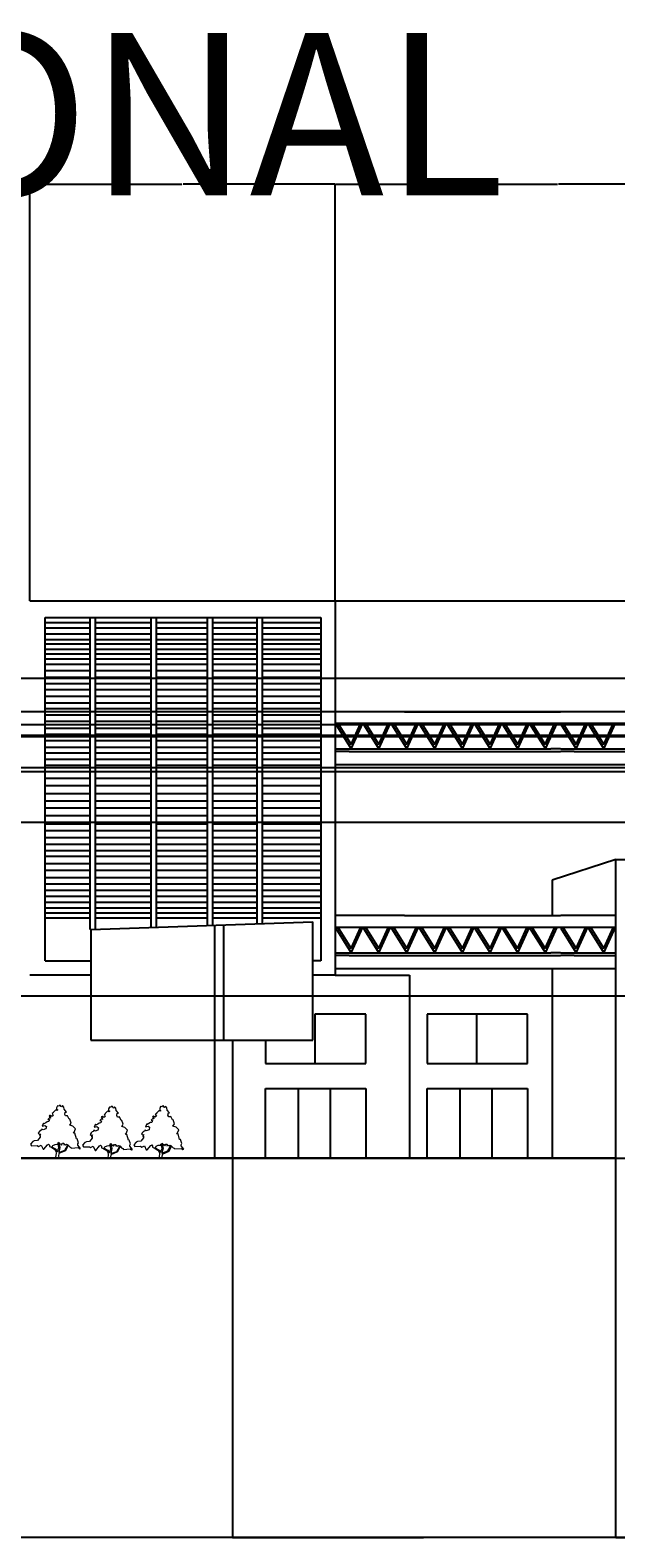
# Model space of a CAD drawing. Units: inches. Extents: x -2248 to 2617, y -128 to 922.
# Tile 5 of 7: x 413 to 820, y -128 to 922. Entities that reach past the tile are written whole.
import ezdxf

# ---------------------------------------------------------------- set-up
doc = ezdxf.new("R2010")
doc.units = ezdxf.units.IN
doc.header["$MEASUREMENT"] = 0
for name, color, linetype, lineweight in [('A-ANNO-DIMS', 2, 'Continuous', 18), ('A-ANNO-TEXT', 7, 'Continuous', 25), ('A-ELEV', 7, 'Continuous', 25), ('L-PLNT', 3, 'Continuous', 18)]:
    doc.layers.add(name, color=color, linetype=linetype, lineweight=lineweight)
doc.styles.get("Standard").update_dxf_attribs({"font": 'arial.ttf'})
doc.dimstyles.get("Standard").update_dxf_attribs({"dimtxt": 0.18, "dimasz": 0.18, "dimexe": 0.18, "dimexo": 0.0625, "dimgap": 0.09, "dimtad": 0, "dimtih": 1, "dimtoh": 1, "dimdec": 4, "dimzin": 0, "dimdsep": 46, "dimtxsty": 'Standard', "dimcen": 0.09, "dimadec": 0, "dimazin": 0, "dimtfac": 1, "dimtdec": 4, "dimtofl": 0, "dimtmove": 0, "dimatfit": 3, "dimfxl": 1, "dimtolj": 1, "dimtzin": 0, "dimarcsym": 0})

# ---------------------------------------------------------------- blocks, each defined once
blk = doc.blocks.new('*U2')
for points in [[(22.0124, 137.721), (18.5475, 141.5624), (15.5282, 138.2446), (13.8028, 139.3505), (13.3714, 142.1153), (11.2148, 143.2214), (8.1954, 140.4564), (4.7447, 141.0094), (2.1567, 136.0326), (2.1567, 131.6088), (5.6074, 129.9499), (3.0193, 128.2909), (0.4313, 130.5029), (-6.9015, 123.3141), (-6.9015, 121.6552), (-9.9208, 119.9963), (-9.0581, 118.3373), (-6.9015, 115.0195), (-10.7835, 112.2546), (-14.6656, 115.0195), (-16.8222, 114.4665), (-17.6849, 112.2546), (-14.6656, 111.7016), (-14.2342, 107.2778), (-17.6065, 107.8307), (-21.5669, 103.9599), (-17.2536, 103.4069), (-18.9789, 97.8771), (-22.8609, 97.3241), (-27.1743, 94.5593), (-32.3504, 91.7944), (-32.7817, 94.0063), (-36.6638, 85.7116), (-29.7624, 87.3705), (-25.449, 84.6056), (-26.743, 77.9699), (-34.507, 75.205), (-37.9578, 77.4169), (-39.2518, 74.099), (-42.2711, 73.5461), (-44.8592, 70.2282), (-47.8786, 66.3574), (-43.9965, 63.0395), (-41.4085, 64.6985), (-44.3346, 59.8898), (-42.2089, 60.1377), (-42.5159, 55.7849), (-49.6039, 46.4502), (-58.2307, 45.8972), (-62.1127, 43.6853), (-68.5828, 36.4966), (-65.9947, 32.0727), (-50.0352, 32.6257), (-47.0159, 30.4138), (-39.6831, 33.7317), (-34.507, 22.6721), (-32.3504, 22.6721), (-22.4296, 34.8376), (-19.4102, 36.4966), (-17.2536, 33.7317), (-17.2536, 29.8608), (-13.8028, 28.7549), (-9.0581, 28.7549), (-7.3328, 32.6257), (-1.7254, 35.3906), (3.8821, 35.9436), (6.4701, 38.1555), (6.9014, 38.7085), (8.1954, 41.4734), (9.9208, 40.3674), (11.2148, 35.9436), (14.2341, 37.6025), (15.0968, 36.4966), (15.9595, 33.7317), (18.9789, 38.7085), (21.9982, 38.7085), (23.2922, 36.4966), (21.9982, 34.2847), (25.4489, 35.3906), (26.743, 33.7317), (29.7623, 35.9436), (32.7817, 34.8376), (38.8204, 28.7549), (41.4084, 27.6489), (43.5651, 25.437), (61.6813, 27.0959), (65.132, 23.7781), (67.7201, 24.884), (60.8186, 33.7317), (60.3873, 37.0495), (62.544, 40.3674), (58.662, 50.874), (56.5053, 50.874), (52.1919, 66.3574), (47.8785, 66.9103), (50.4665, 69.1222), (53.9172, 77.9699), (47.0158, 85.1586), (38.3891, 87.9235), (42.2711, 94.0063)], [(42.2711, 94.0063), (38.8204, 104.5129), (36.6637, 104.5129), (32.3503, 113.9135), (29.7623, 113.3605), (26.743, 113.3605), (24.5862, 117.7844), (25.8802, 123.8671), (29.331, 123.8671), (22.8609, 131.6088), (21.9982, 137.6916)], [(-12.9401, 28.7549), (-2.588, 22.1191), (0.8626, 17.6953), (1.7253, 11.6125), (0, 0)], [(-9.9208, 28.2019), (0, 23.2251), (3.4507, 19.9072), (4.7447, 15.4834), (8.6267, 27.0959), (6.4701, 37.6025)], [(34.5071, 33.1787), (27.1743, 18.2483), (9.0581, 10.5066), (7.7641, 3.8708), (8.1954, 0)], [(8.1954, 40.3674), (11.2148, 27.6489), (8.1954, 13.8245), (24.5862, 19.9072), (32.7817, 34.2847)]]:
    blk.add_lwpolyline(points)
blk = doc.blocks.new('*D16')
at = {"layer": 'A-ANNO-DIMS', "color": 0, "lineweight": -2, "transparency": 16777216}
for p, q in [((45.9, 438.4), (2616.5, 438.4)), ((2616.3, 438.3), (2616.3, 287.6)), ((2616.3, 136.6), (2616.3, 287.3)), ((45.9, 136.5), (2616.5, 136.5))]:
    blk.add_line(p, q, dxfattribs=at)
at = {"layer": 'A-ANNO-DIMS', "color": 0, "transparency": 16777216}
for points in [[(2616.2, 438.3), (2616.3, 438.3), (2616.3, 438.4)], [(2616.2, 136.6), (2616.3, 136.6), (2616.3, 136.5)]]:
    blk.add_solid(points, dxfattribs=at)
at = {"layer": 'Defpoints', "color": 0, "transparency": 16777216}
for p in [(45.8, 438.4), (45.8, 136.5), (2616.3, 136.5)]:
    blk.add_point(p, dxfattribs=at)
at = {"layer": 'A-ANNO-DIMS', "color": 0, "transparency": 16777216, "insert": (2616.3, 287.4), "char_height": 0.18, "attachment_point": 5}
blk.add_mtext('\\A1;302', dxfattribs=at)
blk = doc.blocks.new('*D17')
at = {"layer": 'A-ANNO-DIMS', "color": 0, "lineweight": -2, "transparency": 16777216}
for p, q in [((625.1, 524.3), (2616.5, 524.3)), ((2616.3, 524.1), (2616.3, 330.6)), ((2616.3, 136.6), (2616.3, 330.2)), ((553.6, 136.5), (2616.5, 136.5))]:
    blk.add_line(p, q, dxfattribs=at)
at = {"layer": 'A-ANNO-DIMS', "color": 0, "transparency": 16777216}
for points in [[(2616.2, 524.1), (2616.3, 524.1), (2616.3, 524.3)], [(2616.2, 136.6), (2616.3, 136.6), (2616.3, 136.5)]]:
    blk.add_solid(points, dxfattribs=at)
at = {"layer": 'Defpoints', "color": 0, "transparency": 16777216}
for p in [(625.1, 524.3), (553.6, 136.5), (2616.3, 136.5)]:
    blk.add_point(p, dxfattribs=at)
at = {"layer": 'A-ANNO-DIMS', "color": 0, "transparency": 16777216, "insert": (2616.3, 330.4), "char_height": 0.18, "attachment_point": 5}
blk.add_mtext('\\A1;387.9', dxfattribs=at)
blk = doc.blocks.new('*D20')
at = {"layer": 'A-ANNO-DIMS', "color": 0, "lineweight": -2, "transparency": 16777216}
for p, q in [((-1595.3, 429.9), (2616.5, 429.9)), ((2616.3, 429.7), (2616.3, 417.9)), ((2616.3, 405.8), (2616.3, 417.5)), ((-1653.9, 405.6), (2616.5, 405.6))]:
    blk.add_line(p, q, dxfattribs=at)
at = {"layer": 'A-ANNO-DIMS', "color": 0, "transparency": 16777216}
for points in [[(2616.2, 429.7), (2616.3, 429.7), (2616.3, 429.9)], [(2616.2, 405.8), (2616.3, 405.8), (2616.3, 405.6)]]:
    blk.add_solid(points, dxfattribs=at)
at = {"layer": 'Defpoints', "color": 0, "transparency": 16777216}
for p in [(-1595.4, 429.9), (-1654, 405.6), (2616.3, 405.6)]:
    blk.add_point(p, dxfattribs=at)
at = {"layer": 'A-ANNO-DIMS', "color": 0, "transparency": 16777216, "insert": (2616.3, 417.7), "char_height": 0.18, "attachment_point": 5}
blk.add_mtext('\\A1;24.3', dxfattribs=at)
blk = doc.blocks.new('*D21')
at = {"layer": 'A-ANNO-DIMS', "color": 0, "lineweight": -2, "transparency": 16777216}
for p, q in [((-1125.3, 470.6), (2616.5, 470.6)), ((2616.3, 470.4), (2616.3, 451)), ((2616.3, 431.1), (2616.3, 450.6)), ((-1257.9, 430.9), (2616.5, 430.9))]:
    blk.add_line(p, q, dxfattribs=at)
at = {"layer": 'A-ANNO-DIMS', "color": 0, "transparency": 16777216}
for points in [[(2616.2, 470.4), (2616.3, 470.4), (2616.3, 470.6)], [(2616.2, 431.1), (2616.3, 431.1), (2616.3, 430.9)]]:
    blk.add_solid(points, dxfattribs=at)
at = {"layer": 'Defpoints', "color": 0, "transparency": 16777216}
for p in [(-1125.4, 470.6), (-1258, 430.9), (2616.3, 430.9)]:
    blk.add_point(p, dxfattribs=at)
at = {"layer": 'A-ANNO-DIMS', "color": 0, "transparency": 16777216, "insert": (2616.3, 450.8), "char_height": 0.18, "attachment_point": 5}
blk.add_mtext('\\A1;39.705', dxfattribs=at)
blk = doc.blocks.new('*D22')
at = {"layer": 'A-ANNO-DIMS', "color": 0, "lineweight": -2, "transparency": 16777216}
for p, q in [((-733.3, 408.4), (2616.5, 408.4)), ((2616.3, 408.2), (2616.3, 329.1)), ((2616.3, 249.6), (2616.3, 328.7)), ((-719.1, 249.4), (2616.5, 249.4))]:
    blk.add_line(p, q, dxfattribs=at)
at = {"layer": 'A-ANNO-DIMS', "color": 0, "transparency": 16777216}
for points in [[(2616.2, 408.2), (2616.3, 408.2), (2616.3, 408.4)], [(2616.2, 249.6), (2616.3, 249.6), (2616.3, 249.4)]]:
    blk.add_solid(points, dxfattribs=at)
at = {"layer": 'Defpoints', "color": 0, "transparency": 16777216}
for p in [(-733.4, 408.4), (-719.2, 249.4), (2616.3, 249.4)]:
    blk.add_point(p, dxfattribs=at)
at = {"layer": 'A-ANNO-DIMS', "color": 0, "transparency": 16777216, "insert": (2616.3, 328.9), "char_height": 0.18, "attachment_point": 5}
blk.add_mtext('\\A1;159.02', dxfattribs=at)
blk = doc.blocks.new('*D23')
at = {"layer": 'A-ANNO-DIMS', "color": 0, "lineweight": -2, "transparency": 16777216}
for p, q in [((-719.1, 249.4), (2616.5, 249.4)), ((2616.3, 249.2), (2616.3, 193.1)), ((2616.3, 136.6), (2616.3, 192.7)), ((-719.1, 136.5), (2616.5, 136.5))]:
    blk.add_line(p, q, dxfattribs=at)
at = {"layer": 'A-ANNO-DIMS', "color": 0, "transparency": 16777216}
for points in [[(2616.2, 249.2), (2616.3, 249.2), (2616.3, 249.4)], [(2616.2, 136.6), (2616.3, 136.6), (2616.3, 136.5)]]:
    blk.add_solid(points, dxfattribs=at)
at = {"layer": 'Defpoints', "color": 0, "transparency": 16777216}
for p in [(-719.2, 249.4), (-719.2, 136.5), (2616.3, 136.5)]:
    blk.add_point(p, dxfattribs=at)
at = {"layer": 'A-ANNO-DIMS', "color": 0, "transparency": 16777216, "insert": (2616.3, 192.9), "char_height": 0.18, "attachment_point": 5}
blk.add_mtext('\\A1;112.94', dxfattribs=at)
blk = doc.blocks.new('*D24')
at = {"layer": 'A-ANNO-DIMS', "color": 0, "lineweight": -2, "transparency": 16777216}
for p, q in [((-316.1, 370.3), (2616.5, 370.3)), ((2616.3, 370.1), (2616.3, 253.6)), ((2616.3, 136.6), (2616.3, 253.2)), ((-159.8, 136.5), (2616.5, 136.5))]:
    blk.add_line(p, q, dxfattribs=at)
at = {"layer": 'A-ANNO-DIMS', "color": 0, "transparency": 16777216}
for points in [[(2616.2, 370.1), (2616.3, 370.1), (2616.3, 370.3)], [(2616.2, 136.6), (2616.3, 136.6), (2616.3, 136.5)]]:
    blk.add_solid(points, dxfattribs=at)
at = {"layer": 'Defpoints', "color": 0, "transparency": 16777216}
for p in [(-316.2, 370.3), (-159.9, 136.5), (2616.3, 136.5)]:
    blk.add_point(p, dxfattribs=at)
at = {"layer": 'A-ANNO-DIMS', "color": 0, "transparency": 16777216, "insert": (2616.3, 253.4), "char_height": 0.18, "attachment_point": 5}
blk.add_mtext('\\A1;233.87', dxfattribs=at)
blk = doc.blocks.new('*D31')
at = {"layer": 'A-ANNO-DIMS', "color": 0, "lineweight": -2, "transparency": 16777216}
for p, q in [((934.8, 447.2), (-2247.7, 447.2)), ((-2247.5, 447), (-2247.5, 292)), ((-2247.5, 136.6), (-2247.5, 291.6)), ((820, 136.5), (-2247.7, 136.5))]:
    blk.add_line(p, q, dxfattribs=at)
at = {"layer": 'A-ANNO-DIMS', "color": 0, "transparency": 16777216}
for points in [[(-2247.5, 447), (-2247.5, 447), (-2247.5, 447.2)], [(-2247.5, 136.6), (-2247.5, 136.6), (-2247.5, 136.5)]]:
    blk.add_solid(points, dxfattribs=at)
at = {"layer": 'Defpoints', "color": 0, "transparency": 16777216}
for p in [(934.9, 447.2), (-2247.5, 136.5), (820.1, 136.5)]:
    blk.add_point(p, dxfattribs=at)
at = {"layer": 'A-ANNO-DIMS', "color": 0, "transparency": 16777216, "insert": (-2247.5, 291.8), "char_height": 0.18, "attachment_point": 5}
blk.add_mtext('\\A1;310.7', dxfattribs=at)
blk = doc.blocks.new('*D33')
at = {"layer": 'A-ANNO-DIMS', "color": 0, "lineweight": -2, "transparency": 16777216}
for p, q in [((2393, 136.4), (2393, -127.9)), ((-2024.3, 122), (-2024.3, -127.9)), ((-2024.1, -127.7), (184, -127.7)), ((2392.8, -127.7), (184.7, -127.7))]:
    blk.add_line(p, q, dxfattribs=at)
at = {"layer": 'A-ANNO-DIMS', "color": 0, "transparency": 16777216}
for points in [[(-2024.1, -127.6), (-2024.1, -127.7), (-2024.3, -127.7)], [(2392.8, -127.6), (2392.8, -127.7), (2393, -127.7)]]:
    blk.add_solid(points, dxfattribs=at)
at = {"layer": 'Defpoints', "color": 0, "transparency": 16777216}
for p in [(2393, 136.5), (-2024.3, 122.1), (2393, -127.7)]:
    blk.add_point(p, dxfattribs=at)
at = {"layer": 'A-ANNO-DIMS', "color": 0, "transparency": 16777216, "insert": (184.4, -127.7), "char_height": 0.18, "attachment_point": 5}
blk.add_mtext('\\A1;4417', dxfattribs=at)
blk = doc.blocks.new('*D49')
at = {"layer": 'A-ANNO-DIMS', "color": 0, "lineweight": -2, "transparency": 16777216}
for p, q in [((412.6, 524.4), (412.6, 814.7)), ((412.8, 814.5), (518.4, 814.5)), ((624.9, 814.5), (519.3, 814.5)), ((625.1, 524.4), (625.1, 814.7))]:
    blk.add_line(p, q, dxfattribs=at)
at = {"layer": 'A-ANNO-DIMS', "color": 0, "transparency": 16777216}
for points in [[(412.8, 814.5), (412.8, 814.5), (412.6, 814.5)], [(624.9, 814.5), (624.9, 814.5), (625.1, 814.5)]]:
    blk.add_solid(points, dxfattribs=at)
at = {"layer": 'Defpoints', "color": 0, "transparency": 16777216}
for p in [(625.1, 814.5), (412.6, 524.3), (625.1, 524.3)]:
    blk.add_point(p, dxfattribs=at)
at = {"layer": 'A-ANNO-DIMS', "color": 0, "transparency": 16777216, "insert": (518.8, 814.5), "char_height": 0.18, "attachment_point": 5}
blk.add_mtext('\\A1;212.44', dxfattribs=at)
blk = doc.blocks.new('*D50')
at = {"layer": 'A-ANNO-DIMS', "color": 0, "lineweight": -2, "transparency": 16777216}
for p, q in [((625.1, 524.4), (625.1, 814.7)), ((625.2, 814.5), (779.6, 814.5)), ((934.7, 814.5), (780.4, 814.5)), ((934.9, 591.3), (934.9, 814.7))]:
    blk.add_line(p, q, dxfattribs=at)
at = {"layer": 'A-ANNO-DIMS', "color": 0, "transparency": 16777216}
for points in [[(625.2, 814.5), (625.2, 814.5), (625.1, 814.5)], [(934.7, 814.5), (934.7, 814.5), (934.9, 814.5)]]:
    blk.add_solid(points, dxfattribs=at)
at = {"layer": 'Defpoints', "color": 0, "transparency": 16777216}
for p in [(934.9, 814.5), (934.9, 591.3), (625.1, 524.3)]:
    blk.add_point(p, dxfattribs=at)
at = {"layer": 'A-ANNO-DIMS', "color": 0, "transparency": 16777216, "insert": (780, 814.5), "char_height": 0.18, "attachment_point": 5}
blk.add_mtext('\\A1;309.8', dxfattribs=at)
blk = doc.blocks.new('*D56')
at = {"layer": 'A-ANNO-DIMS', "color": 0, "lineweight": -2, "transparency": 16777216}
for p, q in [((553.6, 136.4), (553.6, -127.9)), ((820.1, 136.4), (820.1, -127.9)), ((553.7, -127.7), (686.4, -127.7)), ((819.9, -127.7), (687.3, -127.7))]:
    blk.add_line(p, q, dxfattribs=at)
at = {"layer": 'A-ANNO-DIMS', "color": 0, "transparency": 16777216}
for points in [[(553.7, -127.6), (553.7, -127.7), (553.6, -127.7)], [(819.9, -127.6), (819.9, -127.7), (820.1, -127.7)]]:
    blk.add_solid(points, dxfattribs=at)
at = {"layer": 'Defpoints', "color": 0, "transparency": 16777216}
for p in [(553.6, 136.5), (820.1, 136.5), (820.1, -127.7)]:
    blk.add_point(p, dxfattribs=at)
at = {"layer": 'A-ANNO-DIMS', "color": 0, "transparency": 16777216, "insert": (686.8, -127.7), "char_height": 0.18, "attachment_point": 5}
blk.add_mtext('\\A1;266.53', dxfattribs=at)
blk = doc.blocks.new('*D57')
at = {"layer": 'A-ANNO-DIMS', "color": 0, "lineweight": -2, "transparency": 16777216}
for p, q in [((820.1, 136.4), (820.1, -127.9)), ((1112.5, 136.4), (1112.5, -127.9)), ((820.3, -127.7), (965.9, -127.7)), ((1112.3, -127.7), (966.7, -127.7))]:
    blk.add_line(p, q, dxfattribs=at)
at = {"layer": 'A-ANNO-DIMS', "color": 0, "transparency": 16777216}
for points in [[(820.3, -127.6), (820.3, -127.7), (820.1, -127.7)], [(1112.3, -127.6), (1112.3, -127.7), (1112.5, -127.7)]]:
    blk.add_solid(points, dxfattribs=at)
at = {"layer": 'Defpoints', "color": 0, "transparency": 16777216}
for p in [(820.1, 136.5), (1112.5, 136.5), (1112.5, -127.7)]:
    blk.add_point(p, dxfattribs=at)
at = {"layer": 'A-ANNO-DIMS', "color": 0, "transparency": 16777216, "insert": (966.3, -127.7), "char_height": 0.18, "attachment_point": 5}
blk.add_mtext('\\A1;292.4', dxfattribs=at)

msp = doc.modelspace()

# ---------------------------------------------------------------- linework, layer by layer
at = {"layer": 'A-ELEV'}
for p, q in [((412.6205, 524.3284), (625.0568, 524.3284)), ((625.0568, 524.3284), (625.0568, 263.9212)), ((423.3579, 273.805), (423.3579, 512.8278)), ((423.3579, 512.8278), (615.0792, 512.8278)), ((423.3579, 509.3192), (454.6069, 509.3192)), ((423.3579, 505.6069), (454.6069, 505.6069)), ((454.6069, 295.6011), (454.6069, 512.8278)), ((458.3874, 295.6011), (458.3874, 512.8278)), ((458.3874, 509.3192), (496.9482, 509.3192)), ((458.3874, 505.6069), (496.9482, 505.6069)), ((496.9482, 297.06), (496.9482, 512.8278)), ((500.7286, 297.1918), (500.7286, 512.8278)), ((500.7286, 509.3192), (536.2651, 509.3192)), ((500.7286, 505.6069), (536.2651, 505.6069)), ((536.2651, 298.4299), (536.2651, 512.8278)), ((540.0455, 298.5616), (540.0455, 512.8278)), ((540.0455, 509.3192), (570.6674, 509.3192)), ((540.0455, 505.6069), (570.6674, 505.6069)), ((570.6674, 299.6286), (570.6674, 512.8278)), ((574.4478, 299.7603), (574.4478, 512.8278)), ((574.4478, 509.3192), (615.0792, 509.3192)), ((574.4478, 505.6069), (615.0792, 505.6069)), ((615.0792, 512.8278), (615.0792, 273.805)), ((423.3579, 501.5233), (454.6069, 501.5233)), ((423.3579, 497.4397), (454.6069, 497.4397)), ((423.3579, 494.4698), (454.6069, 494.4698)), ((458.3874, 501.5233), (496.9482, 501.5233)), ((458.3874, 497.4397), (496.9482, 497.4397)), ((458.3874, 494.4698), (496.9482, 494.4698)), ((500.7286, 501.5233), (536.2651, 501.5233)), ((500.7286, 497.4397), (536.2651, 497.4397)), ((500.7286, 494.4698), (536.2651, 494.4698)), ((540.0455, 501.5233), (570.6674, 501.5233)), ((540.0455, 497.4397), (570.6674, 497.4397)), ((540.0455, 494.4698), (570.6674, 494.4698)), ((574.4478, 501.5233), (615.0792, 501.5233)), ((574.4478, 497.4397), (615.0792, 497.4397)), ((574.4478, 494.4698), (615.0792, 494.4698)), ((423.3579, 490.7574), (454.6069, 490.7574)), ((423.3579, 487.4163), (454.6069, 487.4163)), ((423.3579, 483.9906), (454.6069, 483.9906)), ((458.3874, 490.7574), (496.9482, 490.7574)), ((458.3874, 487.4163), (496.9482, 487.4163)), ((458.3874, 483.9906), (496.9482, 483.9906)), ((500.7286, 490.7574), (536.2651, 490.7574)), ((500.7286, 487.4163), (536.2651, 487.4163)), ((500.7286, 483.9906), (536.2651, 483.9906)), ((540.0455, 490.7574), (570.6674, 490.7574)), ((540.0455, 487.4163), (570.6674, 487.4163)), ((540.0455, 483.9906), (570.6674, 483.9906)), ((574.4478, 490.7574), (615.0792, 490.7574)), ((574.4478, 487.4163), (615.0792, 487.4163)), ((574.4478, 483.9906), (615.0792, 483.9906)), ((423.3579, 480.1939), (454.6069, 480.1939)), ((423.3579, 475.9079), (454.6069, 475.9079)), ((458.3874, 480.1939), (496.9482, 480.1939)), ((458.3874, 475.9079), (496.9482, 475.9079)), ((500.7286, 480.1939), (536.2651, 480.1939)), ((500.7286, 475.9079), (536.2651, 475.9079)), ((540.0455, 480.1939), (570.6674, 480.1939)), ((540.0455, 475.9079), (570.6674, 475.9079)), ((574.4478, 480.1939), (615.0792, 480.1939)), ((574.4478, 475.9079), (615.0792, 475.9079)), ((423.3579, 471.14), (454.6069, 471.14)), ((423.3579, 466.7591), (454.6069, 466.7591)), ((423.3579, 462.6207), (454.6069, 462.6207)), ((458.3874, 471.14), (496.9482, 471.14)), ((458.3874, 466.7591), (496.9482, 466.7591)), ((458.3874, 462.6207), (496.9482, 462.6207)), ((500.7286, 471.14), (536.2651, 471.14)), ((500.7286, 466.7591), (536.2651, 466.7591)), ((500.7286, 462.6207), (536.2651, 462.6207)), ((540.0455, 471.14), (570.6674, 471.14)), ((540.0455, 466.7591), (570.6674, 466.7591)), ((540.0455, 462.6207), (570.6674, 462.6207)), ((574.4478, 471.14), (615.0792, 471.14)), ((574.4478, 466.7591), (615.0792, 466.7591)), ((574.4478, 462.6207), (615.0792, 462.6207)), ((423.3579, 458.0938), (454.6069, 458.0938)), ((423.3579, 453.4208), (454.6069, 453.4208)), ((458.3874, 458.0938), (496.9482, 458.0938)), ((458.3874, 453.4208), (496.9482, 453.4208)), ((500.7286, 458.0938), (536.2651, 458.0938)), ((500.7286, 453.4208), (536.2651, 453.4208)), ((540.0455, 458.0938), (570.6674, 458.0938)), ((540.0455, 453.4208), (570.6674, 453.4208)), ((574.4478, 458.0938), (615.0792, 458.0938)), ((574.4478, 453.4208), (615.0792, 453.4208)), ((423.3579, 449.332), (454.6069, 449.332)), ((423.3579, 445.0971), (454.6069, 445.0971)), ((458.3874, 449.332), (496.9482, 449.332)), ((458.3874, 445.0971), (496.9482, 445.0971)), ((500.7286, 449.332), (536.2651, 449.332)), ((500.7286, 445.0971), (536.2651, 445.0971)), ((540.0455, 449.332), (570.6674, 449.332)), ((540.0455, 445.0971), (570.6674, 445.0971)), ((574.4478, 449.332), (615.0792, 449.332)), ((574.4478, 445.0971), (615.0792, 445.0971)), ((673.2576, 447.1806), (625.4484, 447.1806)), ((673.2576, 447.1806), (781.8576, 447.1806)), ((778.3364, 447.1806), (781.8576, 447.1806)), ((829.7811, 447.1806), (781.9719, 447.1806)), ((423.3579, 440.5702), (454.6069, 440.5702)), ((423.3579, 435.6996), (454.6069, 435.6996)), ((423.3579, 431.4647), (454.6069, 431.4647)), ((458.3874, 440.5702), (496.9482, 440.5702)), ((458.3874, 435.6996), (496.9482, 435.6996)), ((458.3874, 431.4647), (496.9482, 431.4647)), ((500.7286, 440.5702), (536.2651, 440.5702)), ((500.7286, 435.6996), (536.2651, 435.6996)), ((500.7286, 431.4647), (536.2651, 431.4647)), ((540.0455, 440.5702), (570.6674, 440.5702)), ((540.0455, 435.6996), (570.6674, 435.6996)), ((540.0455, 431.4647), (570.6674, 431.4647)), ((574.4478, 440.5702), (615.0792, 440.5702)), ((574.4478, 435.6996), (615.0792, 435.6996)), ((574.4478, 431.4647), (615.0792, 431.4647)), ((625.4484, 439.2108), (781.8576, 439.2108)), ((625.4484, 438.5274), (636.2254, 421.2778)), ((626.8614, 439.2051), (636.1407, 424.3527)), ((636.1407, 424.3527), (642.8533, 439.2108)), ((636.2254, 421.2778), (644.3265, 439.2094)), ((644.2981, 439.2108), (655.5021, 421.2778)), ((646.138, 439.2051), (655.4174, 424.3527)), ((655.4174, 424.3527), (662.13, 439.2108)), ((655.5021, 421.2778), (663.6032, 439.2094)), ((663.775, 439.2108), (674.979, 421.2778)), ((665.615, 439.2051), (674.8943, 424.3527)), ((674.8943, 424.3527), (681.6069, 439.2108)), ((674.979, 421.2778), (683.0801, 439.2094)), ((683.1947, 439.2108), (694.3987, 421.2778)), ((685.0346, 439.2051), (694.314, 424.3527)), ((694.314, 424.3527), (701.0266, 439.2108)), ((694.3987, 421.2778), (702.4998, 439.2094)), ((702.4816, 439.2108), (713.6856, 421.2778)), ((704.3216, 439.2051), (713.6009, 424.3527)), ((713.6009, 424.3527), (720.3135, 439.2108)), ((713.6856, 421.2778), (721.7867, 439.2094)), ((721.7685, 439.2108), (732.9725, 421.2778)), ((723.6085, 439.2051), (732.8878, 424.3527)), ((732.8878, 424.3527), (739.6004, 439.2108)), ((732.9725, 421.2778), (741.0736, 439.2094)), ((740.9081, 439.2108), (752.1122, 421.2778)), ((742.7481, 439.2051), (752.0275, 424.3527)), ((752.0275, 424.3527), (758.74, 439.2108)), ((752.1122, 421.2778), (760.2133, 439.2094)), ((760.1001, 439.2108), (771.3041, 421.2778)), ((761.94, 439.2051), (771.2194, 424.3527)), ((771.2194, 424.3527), (777.932, 439.2108)), ((771.3041, 421.2778), (779.4052, 439.2094)), ((781.9719, 439.2108), (938.3811, 439.2108)), ((781.9719, 438.5274), (792.7489, 421.2778)), ((783.3849, 439.2051), (792.6642, 424.3527)), ((792.6642, 424.3527), (799.3768, 439.2108)), ((792.7489, 421.2778), (800.85, 439.2094)), ((800.8216, 439.2108), (812.0256, 421.2778)), ((802.6615, 439.2051), (811.9409, 424.3527)), ((811.9409, 424.3527), (818.6535, 439.2108)), ((812.0256, 421.2778), (820.1267, 439.2094)), ((423.3579, 427.0838), (454.6069, 427.0838)), ((423.3579, 422.5569), (454.6069, 422.5569)), ((458.3874, 427.0838), (496.9482, 427.0838)), ((458.3874, 422.5569), (496.9482, 422.5569)), ((500.7286, 427.0838), (536.2651, 427.0838)), ((500.7286, 422.5569), (536.2651, 422.5569)), ((540.0455, 427.0838), (570.6674, 427.0838)), ((540.0455, 422.5569), (570.6674, 422.5569)), ((574.4478, 427.0838), (615.0792, 427.0838)), ((574.4478, 422.5569), (615.0792, 422.5569)), ((625.4484, 421.26), (773.5202, 421.26)), ((730.543, 421.26), (730.5579, 421.2274)), ((730.5579, 421.2274), (730.5758, 421.26)), ((773.5202, 421.26), (775.175, 421.26)), ((781.8576, 421.26), (775.175, 421.26)), ((781.9719, 421.26), (930.0437, 421.26)), ((423.3579, 418.6141), (454.6069, 418.6141)), ((423.3579, 414.2332), (454.6069, 414.2332)), ((423.3579, 409.9419), (454.6069, 409.9419)), ((458.3874, 418.6141), (496.9482, 418.6141)), ((458.3874, 414.2332), (496.9482, 414.2332)), ((458.3874, 409.9419), (496.9482, 409.9419)), ((500.7286, 418.6141), (536.2651, 418.6141)), ((500.7286, 414.2332), (536.2651, 414.2332)), ((500.7286, 409.9419), (536.2651, 409.9419)), ((540.0455, 418.6141), (570.6674, 418.6141)), ((540.0455, 414.2332), (570.6674, 414.2332)), ((540.0455, 409.9419), (570.6674, 409.9419)), ((574.4478, 418.6141), (615.0792, 418.6141)), ((574.4478, 414.2332), (615.0792, 414.2332)), ((574.4478, 409.9419), (615.0792, 409.9419)), ((938.3811, 410.2355), (625.2262, 410.2355)), ((634.7533, 419.5059), (625.4484, 419.5059)), ((634.7533, 419.5059), (761.7716, 419.5059)), ((761.7716, 419.5059), (773.5202, 419.5059)), ((773.5202, 419.5059), (781.8576, 419.5059)), ((791.2768, 419.5059), (781.9719, 419.5059)), ((791.2768, 419.5059), (918.2951, 419.5059)), ((423.3579, 405.561), (454.6069, 405.561)), ((423.3579, 401.0341), (454.6069, 401.0341)), ((458.3874, 405.561), (496.9482, 405.561)), ((458.3874, 401.0341), (496.9482, 401.0341)), ((500.7286, 405.561), (536.2651, 405.561)), ((500.7286, 401.0341), (536.2651, 401.0341)), ((540.0455, 405.561), (570.6674, 405.561)), ((540.0455, 401.0341), (570.6674, 401.0341)), ((574.4478, 405.561), (615.0792, 405.561)), ((574.4478, 401.0341), (615.0792, 401.0341)), ((423.3579, 395.9231), (454.6069, 395.9231)), ((423.3579, 390.2279), (454.6069, 390.2279)), ((458.3874, 395.9231), (496.9482, 395.9231)), ((458.3874, 390.2279), (496.9482, 390.2279)), ((500.7286, 395.9231), (536.2651, 395.9231)), ((500.7286, 390.2279), (536.2651, 390.2279)), ((540.0455, 395.9231), (570.6674, 395.9231)), ((540.0455, 390.2279), (570.6674, 390.2279)), ((574.4478, 395.9231), (615.0792, 395.9231)), ((574.4478, 390.2279), (615.0792, 390.2279)), ((423.3579, 385.1943), (454.6069, 385.1943)), ((423.3579, 380.3753), (454.6069, 380.3753)), ((458.3874, 385.1943), (496.9482, 385.1943)), ((458.3874, 380.3753), (496.9482, 380.3753)), ((500.7286, 385.1943), (536.2651, 385.1943)), ((500.7286, 380.3753), (536.2651, 380.3753)), ((540.0455, 385.1943), (570.6674, 385.1943)), ((540.0455, 380.3753), (570.6674, 380.3753)), ((574.4478, 385.1943), (615.0792, 385.1943)), ((574.4478, 380.3753), (615.0792, 380.3753)), ((423.3579, 374.9722), (454.6069, 374.9722)), ((423.3579, 369.131), (454.6069, 369.131)), ((458.3874, 374.9722), (496.9482, 374.9722)), ((458.3874, 369.131), (496.9482, 369.131)), ((500.7286, 374.9722), (536.2651, 374.9722)), ((500.7286, 369.131), (536.2651, 369.131)), ((540.0455, 374.9722), (570.6674, 374.9722)), ((540.0455, 369.131), (570.6674, 369.131)), ((574.4478, 374.9722), (615.0792, 374.9722)), ((574.4478, 369.131), (615.0792, 369.131)), ((423.3579, 364.4269), (454.6069, 364.4269)), ((423.3579, 359.6079), (454.6069, 359.6079)), ((458.3874, 364.4269), (496.9482, 364.4269)), ((458.3874, 359.6079), (496.9482, 359.6079)), ((500.7286, 364.4269), (536.2651, 364.4269)), ((500.7286, 359.6079), (536.2651, 359.6079)), ((540.0455, 364.4269), (570.6674, 364.4269)), ((540.0455, 359.6079), (570.6674, 359.6079)), ((574.4478, 364.4269), (615.0792, 364.4269)), ((574.4478, 359.6079), (615.0792, 359.6079)), ((423.3579, 355.081), (454.6069, 355.081)), ((423.3579, 350.6683), (454.6069, 350.6683)), ((423.3579, 346.5795), (454.6069, 346.5795)), ((458.3874, 355.081), (496.9482, 355.081)), ((458.3874, 350.6683), (496.9482, 350.6683)), ((458.3874, 346.5795), (496.9482, 346.5795)), ((500.7286, 355.081), (536.2651, 355.081)), ((500.7286, 350.6683), (536.2651, 350.6683)), ((500.7286, 346.5795), (536.2651, 346.5795)), ((540.0455, 355.081), (570.6674, 355.081)), ((540.0455, 350.6683), (570.6674, 350.6683)), ((540.0455, 346.5795), (570.6674, 346.5795)), ((574.4478, 355.081), (615.0792, 355.081)), ((574.4478, 350.6683), (615.0792, 350.6683)), ((574.4478, 346.5795), (615.0792, 346.5795)), ((423.3579, 341.6145), (454.6069, 341.6145)), ((423.3579, 336.7955), (454.6069, 336.7955)), ((458.3874, 341.6145), (496.9482, 341.6145)), ((458.3874, 336.7955), (496.9482, 336.7955)), ((500.7286, 341.6145), (536.2651, 341.6145)), ((500.7286, 336.7955), (536.2651, 336.7955)), ((540.0455, 341.6145), (570.6674, 341.6145)), ((540.0455, 336.7955), (570.6674, 336.7955)), ((574.4478, 341.6145), (615.0792, 341.6145)), ((574.4478, 336.7955), (615.0792, 336.7955)), ((820.2683, 344.2299), (775.9122, 329.9027)), ((820.2683, 297.2736), (820.2683, 344.2299)), ((820.2683, 344.2299), (894.0201, 344.2299)), ((423.3579, 331.8305), (454.6069, 331.8305)), ((423.3579, 327.4496), (454.6069, 327.4496)), ((458.3874, 331.8305), (496.9482, 331.8305)), ((458.3874, 327.4496), (496.9482, 327.4496)), ((500.7286, 331.8305), (536.2651, 331.8305)), ((500.7286, 327.4496), (536.2651, 327.4496)), ((540.0455, 331.8305), (570.6674, 331.8305)), ((540.0455, 327.4496), (570.6674, 327.4496)), ((574.4478, 331.8305), (615.0792, 331.8305)), ((574.4478, 327.4496), (615.0792, 327.4496)), ((775.9122, 329.9027), (775.9122, 305.2491)), ((423.3579, 322.9227), (454.6069, 322.9227)), ((423.3579, 318.8338), (454.6069, 318.8338)), ((458.3874, 322.9227), (496.9482, 322.9227)), ((458.3874, 318.8338), (496.9482, 318.8338)), ((500.7286, 322.9227), (536.2651, 322.9227)), ((500.7286, 318.8338), (536.2651, 318.8338)), ((540.0455, 322.9227), (570.6674, 322.9227)), ((540.0455, 318.8338), (570.6674, 318.8338)), ((574.4478, 322.9227), (615.0792, 322.9227)), ((574.4478, 318.8338), (615.0792, 318.8338)), ((423.3579, 314.745), (454.6069, 314.745)), ((423.3579, 310.8022), (454.6069, 310.8022)), ((423.3579, 307.2975), (454.6069, 307.2975)), ((458.3874, 314.745), (496.9482, 314.745)), ((458.3874, 310.8022), (496.9482, 310.8022)), ((458.3874, 307.2975), (496.9482, 307.2975)), ((500.7286, 314.745), (536.2651, 314.745)), ((500.7286, 310.8022), (536.2651, 310.8022)), ((500.7286, 307.2975), (536.2651, 307.2975)), ((540.0455, 314.745), (570.6674, 314.745)), ((540.0455, 310.8022), (570.6674, 310.8022)), ((540.0455, 307.2975), (570.6674, 307.2975)), ((574.4478, 314.745), (615.0792, 314.745)), ((574.4478, 310.8022), (615.0792, 310.8022)), ((574.4478, 307.2975), (615.0792, 307.2975)), ((673.2238, 305.2491), (625.4146, 305.2491)), ((673.2238, 305.2491), (781.8238, 305.2491)), ((778.3027, 305.2491), (781.8238, 305.2491)), ((820.2683, 305.2491), (781.9381, 305.2491)), ((423.3579, 303.736), (454.6069, 303.736)), ((455.0751, 295.6011), (609.5238, 300.9824)), ((455.0751, 295.6011), (455.0751, 218.4692)), ((458.3874, 303.736), (496.9482, 303.736)), ((500.7286, 303.736), (536.2651, 303.736)), ((540.0455, 303.736), (570.6674, 303.736)), ((541.024, 298.5957), (541.024, 218.4692)), ((547.4036, 298.5957), (547.4036, 218.4692)), ((574.4478, 303.736), (615.0792, 303.736)), ((609.5238, 218.4692), (609.5238, 300.9824)), ((625.4146, 297.2793), (781.8238, 297.2793)), ((625.4146, 296.5958), (636.1916, 279.3462)), ((626.8276, 297.2736), (636.107, 282.4211)), ((636.107, 282.4211), (642.8195, 297.2793)), ((636.1916, 279.3462), (644.2928, 297.2779)), ((644.2643, 297.2793), (655.4683, 279.3462)), ((646.1043, 297.2736), (655.3836, 282.4211)), ((655.3836, 282.4211), (662.0962, 297.2793)), ((655.4683, 279.3462), (663.5694, 297.2779)), ((663.7412, 297.2793), (674.9452, 279.3462)), ((665.5812, 297.2736), (674.8605, 282.4211)), ((674.8605, 282.4211), (681.5731, 297.2793)), ((674.9452, 279.3462), (683.0464, 297.2779)), ((683.1609, 297.2793), (694.3649, 279.3462)), ((685.0009, 297.2736), (694.2802, 282.4211)), ((694.2802, 282.4211), (700.9928, 297.2793)), ((694.3649, 279.3462), (702.466, 297.2779)), ((702.4478, 297.2793), (713.6518, 279.3462)), ((704.2878, 297.2736), (713.5671, 282.4211)), ((713.5671, 282.4211), (720.2797, 297.2793)), ((713.6518, 279.3462), (721.7529, 297.2779)), ((721.7347, 297.2793), (732.9387, 279.3462)), ((723.5747, 297.2736), (732.854, 282.4211)), ((732.854, 282.4211), (739.5666, 297.2793)), ((732.9387, 279.3462), (741.0398, 297.2779)), ((740.8744, 297.2793), (752.0784, 279.3462)), ((742.7143, 297.2736), (751.9937, 282.4211)), ((751.9937, 282.4211), (758.7063, 297.2793)), ((752.0784, 279.3462), (760.1795, 297.2779)), ((760.0663, 297.2793), (771.2703, 279.3462)), ((761.9062, 297.2736), (771.1856, 282.4211)), ((771.1856, 282.4211), (777.8982, 297.2793)), ((771.2703, 279.3462), (779.3714, 297.2779)), ((781.9381, 297.2793), (820.2683, 297.2793)), ((781.9381, 296.5958), (792.7151, 279.3462)), ((783.3511, 297.2736), (792.6305, 282.4211)), ((792.6305, 282.4211), (799.343, 297.2793)), ((792.7151, 279.3462), (800.8163, 297.2779)), ((800.7878, 297.2793), (811.9918, 279.3462)), ((802.6278, 297.2736), (811.9071, 282.4211)), ((811.9071, 282.4211), (818.6197, 297.2793)), ((811.9918, 279.3462), (820.0929, 297.2779)), ((820.0929, 297.2779), (820.0929, 136.4519)), ((820.2647, 297.2793), (820.2683, 297.2736)), ((423.3579, 273.805), (455.0751, 273.805)), ((615.0792, 273.805), (609.5238, 273.805)), ((625.4146, 279.3285), (773.4864, 279.3285)), ((634.7196, 277.5744), (625.4146, 277.5744)), ((634.7196, 277.5744), (761.7378, 277.5744)), ((730.5092, 279.3285), (730.5242, 279.2958)), ((730.5242, 279.2958), (730.5421, 279.3285)), ((761.7378, 277.5744), (773.4864, 277.5744)), ((773.4864, 279.3285), (775.1412, 279.3285)), ((773.4864, 277.5744), (781.8238, 277.5744)), ((781.8238, 279.3285), (775.1412, 279.3285)), ((781.9381, 279.3285), (820.0929, 279.3285)), ((791.2431, 277.5744), (781.9381, 277.5744)), ((791.2431, 277.5744), (820.0929, 277.5744)), ((455.0751, 263.9212), (412.6205, 263.9212)), ((625.0568, 263.9212), (609.5238, 263.9212)), ((625.0568, 263.9212), (676.7775, 263.9212)), ((820.0929, 268.3039), (625.1924, 268.3039)), ((676.7775, 263.9212), (676.7775, 136.4519)), ((775.9122, 268.3039), (775.9122, 136.4519)), ((646.3506, 236.7167), (610.9328, 236.7167)), ((610.9328, 236.7167), (610.9328, 202.4298)), ((646.3506, 202.4298), (646.3506, 236.7167)), ((758.799, 236.7167), (689.0532, 236.7167)), ((689.0532, 236.7167), (689.0532, 230.1859)), ((723.3812, 236.7167), (723.3812, 202.4298)), ((758.799, 202.4298), (758.799, 236.7167)), ((689.0532, 230.1859), (689.0532, 202.4298)), ((455.0751, 218.4692), (609.5238, 218.4692)), ((541.024, 218.4692), (541.024, 136.4519)), ((553.5648, 218.4692), (553.5648, 136.4519)), ((576.6048, 218.4692), (576.6048, 202.4298)), ((576.6048, 202.4298), (646.3506, 202.4298)), ((689.0532, 202.4298), (758.799, 202.4298)), ((576.3613, 185.0391), (576.3613, 136.4519)), ((576.6048, 185.0391), (646.3506, 185.0391)), ((599.236, 185.0391), (599.236, 136.4519)), ((621.679, 185.0391), (621.679, 136.4519)), ((646.3506, 185.0391), (646.3506, 136.4519)), ((688.8097, 185.0391), (688.8097, 136.4519)), ((689.0532, 185.0391), (758.799, 185.0391)), ((711.6843, 185.0391), (711.6843, 136.4519)), ((734.1274, 185.0391), (734.1274, 136.4519)), ((758.799, 185.0391), (758.799, 136.4519)), ((-602.3282, 136.4519), (517.5185, 136.4519)), ((517.5185, 136.4519), (894.0201, 136.4519))]:
    msp.add_line(p, q, dxfattribs=at)

# ---------------------------------------------------------------- block references
at = {"layer": 'L-PLNT', "xscale": 0.2549086149440046, "yscale": 0.2549086149440046, "zscale": 0.2549086149440046}
for p in [(430.607, 136.905), (466.7897, 136.096), (502.4324, 136.3657)]:
    msp.add_blockref('*U2', p, dxfattribs=at)

# ---------------------------------------------------------------- texts
at = {"layer": 'A-ANNO-TEXT'}
msp.add_text('MEGA   SCALE   INSTITUTIONAL   COMPLEX    ', height=113.064343, dxfattribs=at).set_placement((-1470.2311, 806.5595))

# ---------------------------------------------------------------- dimensions: what is measured, and where the dimension line sits
at = {"layer": 'A-ANNO-DIMS'}
for base, p1, p2, override, picture, middle in [((625.0568, 814.5189), (412.6205, 524.3284), (625.0568, 524.3284), {"dimdec": 2, "dimlfac": 1, "dimrnd": 0, "dimzin": 0, "dimdsep": 46, "dimlunit": 2}, '*D49', (518.8387, 814.5189)), ((934.8599, 814.5189), (625.0568, 524.3284), (934.8599, 591.2689), {"dimdec": 1, "dimlfac": 1, "dimrnd": 0, "dimzin": 0, "dimdsep": 46, "dimlunit": 2}, '*D50', (779.9584, 814.5189)), ((2393.0245, -127.6745), (-2024.254, 122.0847), (2393.0245, 136.4519), {"dimdec": 0, "dimlfac": 1, "dimrnd": 0, "dimzin": 0, "dimdsep": 46, "dimlunit": 2}, '*D33', (184.3853, -127.6745)), ((820.0929, -127.6745), (553.5648, 136.4519), (820.0929, 136.4519), {"dimdec": 2, "dimlfac": 1, "dimrnd": 0, "dimzin": 0, "dimdsep": 46, "dimlunit": 2}, '*D56', (686.8288, -127.6745)), ((1112.486, -127.6745), (820.0929, 136.4519), (1112.486, 136.4519), {"dimdec": 1, "dimlfac": 1, "dimrnd": 0, "dimzin": 0, "dimdsep": 46, "dimlunit": 2}, '*D57', (966.2895, -127.6745))]:
    dim = msp.add_linear_dim(base=base, p1=p1, p2=p2, dimstyle='Standard', override=override, dxfattribs=at)
    dim.commit()
    dim.dimension.update_dxf_attribs({"geometry": picture, "text_midpoint": middle})
for base, p1, p2, override, picture, middle in [((2616.2745, 136.4519), (625.0568, 524.3284), (553.5648, 136.4519), {"dimdec": 1, "dimlfac": 1, "dimrnd": 0, "dimzin": 0, "dimdsep": 46, "dimlunit": 2}, '*D17', (2616.2745, 330.3901)), ((2616.2745, 430.9238), (-1125.4072, 470.6286), (-1257.9572, 430.9238), {"dimdec": 3, "dimlfac": 1, "dimrnd": 0, "dimzin": 0, "dimdsep": 46, "dimlunit": 2}, '*D21', (2616.2745, 450.7762)), ((-2247.504, 136.4519), (934.8599, 447.1806), (820.0929, 136.4519), {"dimdec": 1, "dimlfac": 1, "dimrnd": 0, "dimzin": 0, "dimdsep": 46, "dimlunit": 2}, '*D31', (-2247.504, 291.8162)), ((2616.2745, 136.4519), (45.827, 438.443), (45.827, 136.4519), {"dimdec": 0, "dimlfac": 1, "dimrnd": 0, "dimzin": 0, "dimdsep": 46, "dimlunit": 2}, '*D16', (2616.2745, 287.4474)), ((2616.2745, 405.5754), (-1595.3791, 429.8743), (-1653.9599, 405.5754), {"dimdec": 1, "dimlfac": 1, "dimrnd": 0, "dimzin": 0, "dimdsep": 46, "dimlunit": 2}, '*D20', (2616.2745, 417.7249)), ((2616.2745, 249.389), (-733.3752, 408.4102), (-719.1936, 249.389), {"dimdec": 2, "dimlfac": 1, "dimrnd": 0, "dimzin": 0, "dimdsep": 46, "dimlunit": 2}, '*D22', (2616.2745, 328.8996)), ((2616.2745, 136.4519), (-316.2025, 370.3211), (-159.9067, 136.4519), {"dimdec": 2, "dimlfac": 1, "dimrnd": 0, "dimzin": 0, "dimdsep": 46, "dimlunit": 2}, '*D24', (2616.2745, 253.3865)), ((2616.2745, 136.4519), (-719.1936, 249.389), (-719.1936, 136.4519), {"dimdec": 2, "dimlfac": 1, "dimrnd": 0, "dimzin": 0, "dimdsep": 46, "dimlunit": 2}, '*D23', (2616.2745, 192.9204))]:
    dim = msp.add_linear_dim(base=base, p1=p1, p2=p2, angle=90, dimstyle='Standard', override=override, dxfattribs=at)
    dim.commit()
    dim.dimension.update_dxf_attribs({"geometry": picture, "text_midpoint": middle})

doc.saveas('drawing.dxf')
